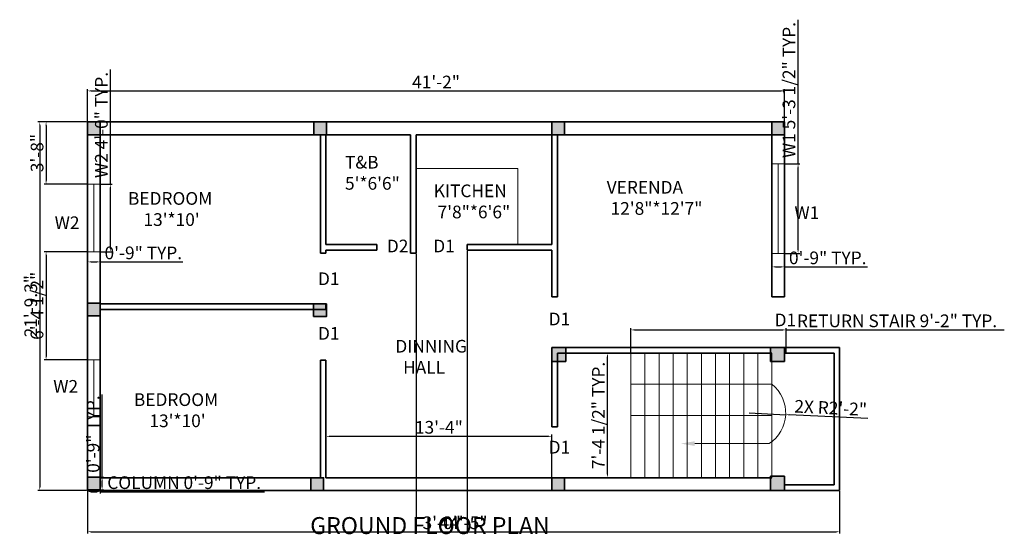
# Model space of a CAD drawing. Units: inches. Extents: x 107 to 1375, y 131 to 922.
# Tile 1 of 4: x 107 to 805, y 131 to 496. Entities that reach past the tile are written whole.
import ezdxf
from ezdxf import colors
from ezdxf.entities.mleader import LeaderData, LeaderLine
from ezdxf.math import Vec2, Vec3

# ---------------------------------------------------------------- set-up
doc = ezdxf.new("R2010")
doc.units = ezdxf.units.IN
for name, color, linetype, lineweight in [('A-ANNO-DIMS', 2, 'Continuous', 13), ('A-ANNO-TEXT', 7, 'Continuous', 18), ('A-ANNO-TITL', 7, 'Continuous', 25), ('A-AREA-IDEN', 7, 'Continuous', 18), ('A-COLS', 7, 'Continuous', 35), ('A-FLOR-FIXT', 8, 'Continuous', 18), ('A-FLOR-STRS', 7, 'Continuous', 18), ('A-GLAZ', 4, 'Continuous', 18), ('A-WALL', 7, 'Continuous', 35)]:
    doc.layers.add(name, color=color, linetype=linetype, lineweight=lineweight)
doc.layers.add('A-COLS-PATT', color=18, linetype='Continuous', lineweight=13, true_color=0x000000)
doc.styles.get("Standard").update_dxf_attribs({"font": 'arial.ttf'})
doc.dimstyles.new('ISO-25', dxfattribs={"dimtxt": 9, "dimasz": 2.5, "dimexe": 1.25, "dimexo": 0.625, "dimtad": 1, "dimlunit": 3, "dimtxsty": 'Standard', "dimcen": 2.5, "dimadec": 0, "dimazin": 0, "dimtfac": 1, "dimtmove": 0, "dimatfit": 3, "dimfxl": 1, "dimarcsym": 0})

# ---------------------------------------------------------------- blocks, each defined once
blk = doc.blocks.new('*D1')
at = {"layer": 'A-ANNO-DIMS', "color": 0, "lineweight": -2, "transparency": 16777216}
for p, q in [((155.4, 423.72), (155.4, 446.38)), ((157.9, 445.13), (646.9, 445.13)), ((649.4, 423.72), (649.4, 446.38))]:
    blk.add_line(p, q, dxfattribs=at)
at = {"layer": 'A-ANNO-DIMS', "color": 0, "transparency": 16777216}
for points in [[(157.9, 445.55), (157.9, 444.72), (155.4, 445.13)], [(646.9, 445.55), (646.9, 444.72), (649.4, 445.13)]]:
    blk.add_solid(points, dxfattribs=at)
at = {"layer": 'Defpoints', "color": 0, "transparency": 16777216}
for p in [(649.4, 445.13), (155.4, 423.09), (649.4, 423.09)]:
    blk.add_point(p, dxfattribs=at)
at = {"layer": 'A-ANNO-DIMS', "color": 0, "transparency": 16777216, "insert": (402.4, 450.28), "char_height": 9, "attachment_point": 5}
blk.add_mtext('41\'-2"', dxfattribs=at)
blk = doc.blocks.new('*D2')
at = {"layer": 'A-ANNO-DIMS', "color": 0, "lineweight": -2, "transparency": 16777216}
for p, q in [((154.77, 423.09), (120.32, 423.09)), ((121.57, 420.59), (121.57, 164.29)), ((154.77, 161.79), (120.32, 161.79))]:
    blk.add_line(p, q, dxfattribs=at)
at = {"layer": 'A-ANNO-DIMS', "color": 0, "transparency": 16777216}
for points in [[(121.15, 420.59), (121.98, 420.59), (121.57, 423.09)], [(121.15, 164.29), (121.98, 164.29), (121.57, 161.79)]]:
    blk.add_solid(points, dxfattribs=at)
at = {"layer": 'Defpoints', "color": 0, "transparency": 16777216}
for p in [(155.4, 423.09), (121.57, 161.79), (155.4, 161.79)]:
    blk.add_point(p, dxfattribs=at)
at = {"layer": 'A-ANNO-DIMS', "color": 0, "transparency": 16777216, "insert": (116.34, 292.44), "char_height": 9, "attachment_point": 5, "rotation": 90}
blk.add_mtext('21\'-9.3"', dxfattribs=at)
blk = doc.blocks.new('COLUMN-10x10')
h = blk.add_hatch(color=256)
h.dxf.hatch_style = 1
h.paths.add_polyline_path([(10, 10), (0, 10), (0, 0), (10, 0)])
for p, q in [((10, 10), (0, 10)), ((0, 10), (0, 0)), ((10, 0), (10, 10)), ((0, 0), (10, 0))]:
    blk.add_line(p, q)
blk = doc.blocks.new('COLUMN-9x9')
h = blk.add_hatch(color=256)
h.dxf.hatch_style = 1
h.paths.add_polyline_path([(9, 9), (0, 9), (0, 0), (9, 0)])
blk.add_lwpolyline([(0, 0), (9, 0), (9, 9), (0, 9)], close=True)
blk = doc.blocks.new('WINDOW-PLAN-W1')
for p, q in [((0, 63.51), (0, 0)), ((0, 63.51), (9, 63.51)), ((4.5, 63.51), (4.5, 0)), ((9, 0), (9, 63.51)), ((0, 0), (9, 0))]:
    blk.add_line(p, q)
blk = doc.blocks.new('WINDOW-PLAN-W2-OFFSET')
for p, q in [((0, 48), (0, 0)), ((0, 48), (9, 48)), ((4.5, 48), (4.5, 7.53)), ((9, 0), (9, 48)), ((0, 7.53), (9, 7.53))]:
    blk.add_line(p, q)
blk = doc.blocks.new('WINDOW-PLAN-W2')
for p, q in [((0, 48), (0, 0)), ((0, 48), (9, 48)), ((4.5, 48), (4.5, 0)), ((9, 0), (9, 48)), ((0, 0), (9, 0))]:
    blk.add_line(p, q)
blk = doc.blocks.new('KITCHEN-COUNTER-L')
for q in [(0, 54), (72, 0)]:
    blk.add_line((72, 54), q)
blk = doc.blocks.new('*D20')
at = {"layer": 'A-ANNO-DIMS', "color": 0, "lineweight": -2, "transparency": 16777216}
for p, q in [((155.4, 161.54), (155.4, 159.56)), ((157.9, 160.81), (161.9, 160.81)), ((164.4, 161.54), (164.4, 159.56)), ((164.4, 160.81), (280.88, 160.81))]:
    blk.add_line(p, q, dxfattribs=at)
at = {"layer": 'A-ANNO-DIMS', "color": 0, "transparency": 16777216}
for points in [[(157.9, 161.23), (157.9, 160.4), (155.4, 160.81)], [(161.9, 161.23), (161.9, 160.4), (164.4, 160.81)]]:
    blk.add_solid(points, dxfattribs=at)
at = {"layer": 'Defpoints', "color": 0, "transparency": 16777216}
for p in [(155.4, 162.16), (164.4, 162.16), (164.4, 160.81)]:
    blk.add_point(p, dxfattribs=at)
at = {"layer": 'A-ANNO-DIMS', "color": 0, "transparency": 16777216, "insert": (223.89, 166.1), "char_height": 9, "attachment_point": 5}
blk.add_mtext('COLUMN 0\'-9" TYP.', dxfattribs=at)
blk = doc.blocks.new('*D21')
at = {"layer": 'A-ANNO-DIMS', "color": 0, "lineweight": -2, "transparency": 16777216}
for p, q in [((165.75, 171.16), (165.75, 229.77)), ((165.02, 171.16), (167, 171.16)), ((165.75, 164.66), (165.75, 168.66)), ((165.02, 162.16), (167, 162.16))]:
    blk.add_line(p, q, dxfattribs=at)
at = {"layer": 'A-ANNO-DIMS', "color": 0, "transparency": 16777216}
for points in [[(165.33, 168.66), (166.16, 168.66), (165.75, 171.16)], [(165.33, 164.66), (166.16, 164.66), (165.75, 162.16)]]:
    blk.add_solid(points, dxfattribs=at)
at = {"layer": 'Defpoints', "color": 0, "transparency": 16777216}
for p in [(164.4, 171.16), (165.75, 171.16), (164.4, 162.16)]:
    blk.add_point(p, dxfattribs=at)
at = {"layer": 'A-ANNO-DIMS', "color": 0, "transparency": 16777216, "insert": (160.53, 201.72), "char_height": 9, "attachment_point": 5, "rotation": 90}
blk.add_mtext('0\'-9" TYP.', dxfattribs=at)
blk = doc.blocks.new('*D24')
at = {"layer": 'A-ANNO-DIMS', "color": 0, "lineweight": -2, "transparency": 16777216}
for p, q in [((658.92, 393.37), (658.92, 495.67)), ((650.02, 393.37), (660.17, 393.37)), ((658.92, 332.36), (658.92, 390.87)), ((650.02, 329.86), (660.17, 329.86))]:
    blk.add_line(p, q, dxfattribs=at)
at = {"layer": 'A-ANNO-DIMS', "color": 0, "transparency": 16777216}
for points in [[(658.51, 390.87), (659.34, 390.87), (658.92, 393.37)], [(658.51, 332.36), (659.34, 332.36), (658.92, 329.86)]]:
    blk.add_solid(points, dxfattribs=at)
at = {"layer": 'Defpoints', "color": 0, "transparency": 16777216}
for p in [(649.4, 393.37), (658.92, 393.37), (649.4, 329.86)]:
    blk.add_point(p, dxfattribs=at)
at = {"layer": 'A-ANNO-DIMS', "color": 0, "transparency": 16777216, "insert": (653.64, 445.77), "char_height": 9, "attachment_point": 5, "rotation": 90}
blk.add_mtext('W1 5\'-3 1/2" TYP.', dxfattribs=at)
blk = doc.blocks.new('*D25')
at = {"layer": 'A-ANNO-DIMS', "color": 0, "lineweight": -2, "transparency": 16777216}
for p, q in [((640.4, 329.24), (640.4, 319.09)), ((649.4, 329.24), (649.4, 319.09)), ((642.9, 320.34), (646.9, 320.34)), ((649.4, 320.34), (708.01, 320.34))]:
    blk.add_line(p, q, dxfattribs=at)
at = {"layer": 'A-ANNO-DIMS', "color": 0, "transparency": 16777216}
for points in [[(642.9, 320.75), (642.9, 319.92), (640.4, 320.34)], [(646.9, 320.75), (646.9, 319.92), (649.4, 320.34)]]:
    blk.add_solid(points, dxfattribs=at)
at = {"layer": 'Defpoints', "color": 0, "transparency": 16777216}
for p in [(640.4, 329.86), (649.4, 329.86), (649.4, 320.34)]:
    blk.add_point(p, dxfattribs=at)
at = {"layer": 'A-ANNO-DIMS', "color": 0, "transparency": 16777216, "insert": (679.95, 325.56), "char_height": 9, "attachment_point": 5}
blk.add_mtext('0\'-9" TYP.', dxfattribs=at)
blk = doc.blocks.new('*D28')
at = {"layer": 'A-ANNO-DIMS', "color": 0, "lineweight": -2, "transparency": 16777216}
for p, q in [((171.6, 379.06), (171.6, 460.39)), ((165.02, 379.06), (172.85, 379.06)), ((171.6, 333.56), (171.6, 376.56)), ((165.02, 331.06), (172.85, 331.06))]:
    blk.add_line(p, q, dxfattribs=at)
at = {"layer": 'A-ANNO-DIMS', "color": 0, "transparency": 16777216}
for points in [[(171.18, 376.56), (172.01, 376.56), (171.6, 379.06)], [(171.18, 333.56), (172.01, 333.56), (171.6, 331.06)]]:
    blk.add_solid(points, dxfattribs=at)
at = {"layer": 'Defpoints', "color": 0, "transparency": 16777216}
for p in [(164.4, 379.06), (171.6, 379.06), (164.4, 331.06)]:
    blk.add_point(p, dxfattribs=at)
at = {"layer": 'A-ANNO-DIMS', "color": 0, "transparency": 16777216, "insert": (166.38, 420.98), "char_height": 9, "attachment_point": 5, "rotation": 90}
blk.add_mtext('W2 4\'-0" TYP.', dxfattribs=at)
blk = doc.blocks.new('*D29')
at = {"layer": 'A-ANNO-DIMS', "color": 0, "lineweight": -2, "transparency": 16777216}
for p, q in [((155.4, 330.44), (155.4, 322.61)), ((164.4, 330.44), (164.4, 322.61)), ((157.9, 323.86), (161.9, 323.86)), ((164.4, 323.86), (223.01, 323.86))]:
    blk.add_line(p, q, dxfattribs=at)
at = {"layer": 'A-ANNO-DIMS', "color": 0, "transparency": 16777216}
for points in [[(157.9, 324.28), (157.9, 323.45), (155.4, 323.86)], [(161.9, 324.28), (161.9, 323.45), (164.4, 323.86)]]:
    blk.add_solid(points, dxfattribs=at)
at = {"layer": 'Defpoints', "color": 0, "transparency": 16777216}
for p in [(155.4, 331.06), (164.4, 331.06), (164.4, 323.86)]:
    blk.add_point(p, dxfattribs=at)
at = {"layer": 'A-ANNO-DIMS', "color": 0, "transparency": 16777216, "insert": (194.95, 329.08), "char_height": 9, "attachment_point": 5}
blk.add_mtext('0\'-9" TYP.', dxfattribs=at)
blk = doc.blocks.new('*D32')
at = {"layer": 'A-ANNO-DIMS', "color": 0, "lineweight": -2, "transparency": 16777216}
for p, q in [((540.4, 259.72), (540.4, 276.86)), ((542.9, 275.61), (648.03, 275.61)), ((650.53, 259.72), (650.53, 276.86)), ((650.53, 275.61), (805.07, 275.61))]:
    blk.add_line(p, q, dxfattribs=at)
at = {"layer": 'A-ANNO-DIMS', "color": 0, "transparency": 16777216}
for points in [[(542.9, 276.03), (542.9, 275.2), (540.4, 275.61)], [(648.03, 276.03), (648.03, 275.2), (650.53, 275.61)]]:
    blk.add_solid(points, dxfattribs=at)
at = {"layer": 'Defpoints', "color": 0, "transparency": 16777216}
for p in [(650.53, 275.61), (540.4, 259.09), (650.53, 259.09)]:
    blk.add_point(p, dxfattribs=at)
at = {"layer": 'A-ANNO-DIMS', "color": 0, "transparency": 16777216, "insert": (729.05, 280.89), "char_height": 9, "attachment_point": 5}
blk.add_mtext('RETURN STAIR 9\'-2" TYP.', dxfattribs=at)
blk = doc.blocks.new('*D33')
at = {"layer": 'A-ANNO-DIMS', "color": 0, "lineweight": -2, "transparency": 16777216}
for p, q in [((539.77, 259.09), (522.63, 259.09)), ((523.88, 173.29), (523.88, 256.59)), ((539.77, 170.79), (522.63, 170.79))]:
    blk.add_line(p, q, dxfattribs=at)
at = {"layer": 'A-ANNO-DIMS', "color": 0, "transparency": 16777216}
for points in [[(523.46, 256.59), (524.29, 256.59), (523.88, 259.09)], [(523.46, 173.29), (524.29, 173.29), (523.88, 170.79)]]:
    blk.add_solid(points, dxfattribs=at)
at = {"layer": 'Defpoints', "color": 0, "transparency": 16777216}
for p in [(523.88, 259.09), (540.4, 259.09), (540.4, 170.79)]:
    blk.add_point(p, dxfattribs=at)
at = {"layer": 'A-ANNO-DIMS', "color": 0, "transparency": 16777216, "insert": (518.6, 214.94), "char_height": 9, "attachment_point": 5, "rotation": 90}
blk.add_mtext('7\'-4 1/2" TYP.', dxfattribs=at)
blk = doc.blocks.new('*D46')
at = {"layer": 'A-ANNO-DIMS', "color": 0, "lineweight": -2, "transparency": 16777216}
for p, q in [((155.4, 161.17), (155.4, 131.19)), ((688.4, 161.17), (688.4, 131.19)), ((157.9, 132.44), (685.9, 132.44))]:
    blk.add_line(p, q, dxfattribs=at)
at = {"layer": 'A-ANNO-DIMS', "color": 0, "transparency": 16777216}
for points in [[(157.9, 132.86), (157.9, 132.02), (155.4, 132.44)], [(685.9, 132.86), (685.9, 132.02), (688.4, 132.44)]]:
    blk.add_solid(points, dxfattribs=at)
at = {"layer": 'Defpoints', "color": 0, "transparency": 16777216}
for p in [(155.4, 161.79), (688.4, 161.79), (688.4, 132.44)]:
    blk.add_point(p, dxfattribs=at)
at = {"layer": 'A-ANNO-DIMS', "color": 0, "transparency": 16777216, "insert": (421.9, 137.64), "char_height": 9, "attachment_point": 5}
blk.add_mtext('44\'-5"', dxfattribs=at)
blk = doc.blocks.new('*D48')
at = {"layer": 'A-ANNO-DIMS', "color": 0, "lineweight": -2, "transparency": 16777216}
for p, q in [((388.4, 329.47), (388.4, 131.19)), ((424.4, 331.47), (424.4, 131.19)), ((390.9, 132.44), (421.9, 132.44))]:
    blk.add_line(p, q, dxfattribs=at)
at = {"layer": 'A-ANNO-DIMS', "color": 0, "transparency": 16777216}
for points in [[(390.9, 132.86), (390.9, 132.02), (388.4, 132.44)], [(421.9, 132.86), (421.9, 132.02), (424.4, 132.44)]]:
    blk.add_solid(points, dxfattribs=at)
at = {"layer": 'Defpoints', "color": 0, "transparency": 16777216}
for p in [(388.4, 330.09), (424.4, 332.09), (424.4, 132.44)]:
    blk.add_point(p, dxfattribs=at)
at = {"layer": 'A-ANNO-DIMS', "color": 0, "transparency": 16777216, "insert": (406.4, 137.66), "char_height": 9, "attachment_point": 5}
blk.add_mtext('3\'-0"', dxfattribs=at)
blk = doc.blocks.new('*D49')
at = {"layer": 'A-ANNO-DIMS', "color": 0, "lineweight": -2, "transparency": 16777216}
for p, q in [((154.77, 423.09), (124.8, 423.09)), ((126.05, 420.59), (126.05, 381.56)), ((154.77, 379.06), (124.8, 379.06))]:
    blk.add_line(p, q, dxfattribs=at)
at = {"layer": 'A-ANNO-DIMS', "color": 0, "transparency": 16777216}
for points in [[(125.63, 420.59), (126.46, 420.59), (126.05, 423.09)], [(125.63, 381.56), (126.46, 381.56), (126.05, 379.06)]]:
    blk.add_solid(points, dxfattribs=at)
at = {"layer": 'Defpoints', "color": 0, "transparency": 16777216}
for p in [(155.4, 423.09), (126.05, 379.06), (155.4, 379.06)]:
    blk.add_point(p, dxfattribs=at)
at = {"layer": 'A-ANNO-DIMS', "color": 0, "transparency": 16777216, "insert": (120.82, 401.08), "char_height": 9, "attachment_point": 5, "rotation": 90}
blk.add_mtext('3\'-8"', dxfattribs=at)
blk = doc.blocks.new('*D50')
at = {"layer": 'A-ANNO-DIMS', "color": 0, "lineweight": -2, "transparency": 16777216}
for p, q in [((154.77, 331.06), (124.8, 331.06)), ((126.05, 328.56), (126.05, 256.86)), ((154.77, 254.36), (124.8, 254.36))]:
    blk.add_line(p, q, dxfattribs=at)
at = {"layer": 'A-ANNO-DIMS', "color": 0, "transparency": 16777216}
for points in [[(125.63, 328.56), (126.46, 328.56), (126.05, 331.06)], [(125.63, 256.86), (126.46, 256.86), (126.05, 254.36)]]:
    blk.add_solid(points, dxfattribs=at)
at = {"layer": 'Defpoints', "color": 0, "transparency": 16777216}
for p in [(155.4, 331.06), (126.05, 254.36), (155.4, 254.36)]:
    blk.add_point(p, dxfattribs=at)
at = {"layer": 'A-ANNO-DIMS', "color": 0, "transparency": 16777216, "insert": (120.77, 292.71), "char_height": 9, "attachment_point": 5, "rotation": 90}
blk.add_mtext('6\'-4 1/2"', dxfattribs=at)
blk = doc.blocks.new('*D55')
at = {"layer": 'A-ANNO-DIMS', "color": 0, "lineweight": -2, "transparency": 16777216}
for p, q in [((324.4, 171.42), (324.4, 201.39)), ((326.9, 200.14), (481.9, 200.14)), ((484.4, 171.42), (484.4, 201.39))]:
    blk.add_line(p, q, dxfattribs=at)
at = {"layer": 'A-ANNO-DIMS', "color": 0, "transparency": 16777216}
for points in [[(326.9, 200.56), (326.9, 199.72), (324.4, 200.14)], [(481.9, 200.56), (481.9, 199.72), (484.4, 200.14)]]:
    blk.add_solid(points, dxfattribs=at)
at = {"layer": 'Defpoints', "color": 0, "transparency": 16777216}
for p in [(484.4, 200.14), (324.4, 170.79), (484.4, 170.79)]:
    blk.add_point(p, dxfattribs=at)
at = {"layer": 'A-ANNO-DIMS', "color": 0, "transparency": 16777216, "insert": (404.4, 205.36), "char_height": 9, "attachment_point": 5}
blk.add_mtext('13\'-4"', dxfattribs=at)
blk = doc.blocks.new('*D79')
at = {"layer": 'A-ANNO-DIMS', "color": 0, "lineweight": -2, "transparency": 16777216}
for p, q in [((624.18, 216.72), (650.14, 215.49)), ((708.35, 212.72), (652.63, 215.37))]:
    blk.add_line(p, q, dxfattribs=at)
at = {"layer": 'A-ANNO-DIMS', "color": 0, "transparency": 16777216}
blk.add_solid([(652.65, 215.79), (652.61, 214.95), (650.14, 215.49)], dxfattribs=at)
at = {"layer": 'Defpoints', "color": 0, "transparency": 16777216}
for p in [(624.18, 216.72), (650.14, 215.49)]:
    blk.add_point(p, dxfattribs=at)
at = {"layer": 'A-ANNO-DIMS', "color": 0, "transparency": 16777216, "insert": (681.99, 219.13), "char_height": 9, "attachment_point": 5, "rotation": 357.27702}
blk.add_mtext('2X R2\'-2"', dxfattribs=at)
blk = doc.blocks.new('STAIR-RETURN-PLAN')
for p, q in [((0, 0), (0, 88.3)), ((10, 0), (10, 88.3)), ((20, 0), (20, 88.3)), ((30, 0), (30, 88.3)), ((40, 0), (40, 88.3)), ((50, 0), (50, 88.3)), ((60, 0), (60, 88.3)), ((70, 0), (70, 88.3)), ((80, 0), (80, 88.3)), ((90, 0), (90, 88.3)), ((100, 0), (100, 88.3)), ((0, 66.24), (100, 66.24)), ((0, 44.15), (100, 44.15))]:
    blk.add_line(p, q)
for start, end in [(303.16419, 51.39065), (236.83581, 237.96095)]:
    blk.add_arc((83.79, 45.93), 25.99, start, end)
ml = blk.add_multileader_mtext('Standard')
ml.set_content('', color=256)
ml.set_leader_properties(color=256)
ml.build(insert=Vec2(0, 0))
ml.multileader.update_dxf_attribs({"arrow_head_size": 10})
ctx = ml.context
ctx.base_point, ctx.arrow_head_size, ctx.plane_origin = Vec3(98, 24.18), 10, Vec3(35.35, 24.18)
notes = []
notes.append((ctx, [(0, (1, 1, 0), (90, 24.18), (1, 0), 8, [(0, [(35.35, 24.18)], 0, [])])]))
ctx.mtext.insert, ctx.mtext.flow_direction = Vec3(100, 26.18), 5
for ctx, leaders in notes:
    for number, flags, end, landing, length, lines in leaders:
        leader = LeaderData()
        leader.index, (leader.has_last_leader_line, leader.has_dogleg_vector, leader.attachment_direction) = number, flags
        leader.last_leader_point, leader.dogleg_vector, leader.dogleg_length = Vec3(end), Vec3(landing), length
        for number, points, colour, breaks in lines:
            line = LeaderLine()
            line.index, line.vertices, line.color, line.breaks = number, Vec3.list(points), colors.encode_raw_color(colour), breaks
            leader.lines.append(line)
        ctx.leaders.append(leader)

msp = doc.modelspace()

# ---------------------------------------------------------------- hatches: boundary and pattern name
at = {"layer": 'A-COLS-PATT'}
h = msp.add_hatch(color=256, dxfattribs=at)
h.dxf.hatch_style = 1
h.paths.add_polyline_path([(164.397, 423.091), (155.397, 423.091), (155.397, 414.091), (164.397, 414.091)])

# ---------------------------------------------------------------- linework, layer by layer
at = {"layer": 'A-COLS'}
msp.add_lwpolyline([(155.397, 414.091), (164.397, 414.091), (164.397, 423.091), (155.397, 423.091)], close=True, dxfattribs=at)
at = {"layer": 'A-WALL'}
for p, q in [((649.397, 423.091), (155.397, 423.091)), ((155.397, 423.091), (155.397, 161.791)), ((649.397, 299.091), (649.397, 423.091)), ((164.397, 414.091), (164.397, 294.091)), ((320.397, 414.091), (164.397, 414.091)), ((320.397, 414.091), (320.397, 330.091)), ((324.397, 414.091), (324.397, 336.091)), ((384.397, 414.091), (324.397, 414.091)), ((384.397, 414.091), (384.397, 330.091)), ((402.397, 414.091), (388.397, 414.091)), ((484.397, 414.091), (388.397, 414.091)), ((388.397, 414.091), (388.397, 330.091)), ((484.397, 414.091), (484.397, 336.091)), ((640.397, 414.091), (488.397, 414.091)), ((488.397, 414.091), (488.397, 299.091)), ((640.397, 299.091), (640.397, 414.091)), ((360.397, 336.091), (324.397, 336.091)), ((360.397, 336.091), (360.397, 332.091)), ((484.397, 336.091), (424.397, 336.091)), ((424.397, 336.091), (424.397, 332.091)), ((320.397, 330.091), (324.397, 330.091)), ((360.397, 332.091), (324.397, 332.091)), ((324.397, 332.091), (324.397, 330.091)), ((384.397, 330.091), (388.397, 330.091)), ((484.397, 332.091), (424.397, 332.091)), ((484.397, 332.091), (484.397, 299.091)), ((324.397, 294.091), (164.397, 294.091)), ((324.397, 294.091), (324.397, 290.091)), ((488.397, 299.091), (484.397, 299.091)), ((640.397, 299.091), (649.397, 299.091)), ((324.397, 290.091), (164.397, 290.091)), ((164.397, 290.091), (164.397, 170.791)), ((640.397, 263.091), (484.397, 263.091)), ((484.397, 263.091), (484.397, 206.791)), ((640.397, 259.091), (488.397, 259.091)), ((488.397, 259.091), (488.397, 206.791)), ((640.397, 263.091), (688.397, 263.091)), ((649.319, 263.091), (649.319, 259.091)), ((649.319, 259.091), (684.397, 259.091)), ((684.397, 259.091), (684.397, 165.791)), ((688.397, 263.091), (688.397, 161.791)), ((324.397, 254.091), (320.397, 254.091)), ((320.397, 254.091), (320.397, 170.791)), ((324.397, 254.091), (324.397, 170.791)), ((484.397, 206.791), (488.397, 206.791)), ((164.397, 170.791), (320.397, 170.791)), ((324.397, 170.791), (640.397, 170.791)), ((155.397, 161.791), (649.397, 161.791)), ((684.397, 165.791), (649.397, 165.791)), ((649.397, 165.791), (649.397, 161.791)), ((688.397, 161.791), (649.397, 161.791))]:
    msp.add_line(p, q, dxfattribs=at)

# ---------------------------------------------------------------- block references
at = {"layer": 'A-COLS'}
for name, p in [('COLUMN-9x9', (315.721, 414.091)), ('COLUMN-9x9', (484.336, 414.091)), ('COLUMN-9x9', (640.354, 414.091)), ('COLUMN-9x9', (155.397, 285.58)), ('COLUMN-9x9', (315.659, 285.091)), ('COLUMN-10x10', (484.397, 253.091)), ('COLUMN-10x10', (639.319, 253.091)), ('COLUMN-9x9', (155.397, 162.165)), ('COLUMN-9x9', (313.71, 161.791)), ('COLUMN-9x9', (484.397, 161.791)), ('COLUMN-10x10', (639.397, 161.791))]:
    msp.add_blockref(name, p, dxfattribs=at)
at = {"layer": 'A-FLOR-FIXT'}
msp.add_blockref('KITCHEN-COUNTER-L', (388.397, 336.091), dxfattribs=at)
at = {"layer": 'A-FLOR-STRS'}
msp.add_blockref('STAIR-RETURN-PLAN', (540.397, 170.791), dxfattribs=at)
at = {"layer": 'A-GLAZ'}
for name, p in [('WINDOW-PLAN-W1', (640.397, 329.862)), ('WINDOW-PLAN-W2', (155.397, 331.064)), ('WINDOW-PLAN-W2-OFFSET', (155.397, 206.359))]:
    msp.add_blockref(name, p, dxfattribs=at)

# ---------------------------------------------------------------- texts
at = {"layer": 'A-ANNO-TEXT', "char_height": 9, "attachment_point": 1}
for s, insert in [('W1', (656.351, 363.214)), ('W2', (132.141, 356.135)), ('D2', (367.525, 339.617)), ('D1', (400.427, 339.617)), ('D1', (318.726, 316.377)), ('D1', (482.182, 287.865)), ('D1', (642.301, 287.194)), ('D1', (318.726, 277.637)), ('W2', (131.147, 240.071)), ('D1', (482.182, 196.943))]:
    msp.add_mtext_dynamic_manual_height_columns(s, width=33.2577, gutter_width=12.5, heights=[0], dxfattribs=dict(at, insert=insert))
at = {"layer": 'A-ANNO-TITL', "insert": (313.216, 142.83), "char_height": 12, "attachment_point": 1}
msp.add_mtext_dynamic_manual_height_columns('GROUND FLOOR PLAN', width=264.80934, gutter_width=12.5, heights=[0], dxfattribs=at)
at = {"layer": 'A-AREA-IDEN', "char_height": 9, "attachment_point": 1}
for s, width, insert in [('T&B\\P5\'*6\'6"', 26.62767, (337.879, 399.061)), ('KITCHEN\\P 7\'8"*6\'6"', 54.9024, (400.742, 378.764)), ('VERENDA \\P 12\'8"*12\'7"', 89.49012, (523.321, 381.268)), ("BEDROOM\\P    13'*10'", 64.41797, (184.073, 373.369)), ('DINNING\\P  HALL ', 53.67099, (373.54, 268.537)), ("BEDROOM\\P    13'*10'", 64.41797, (188.274, 230.643))]:
    msp.add_mtext_dynamic_manual_height_columns(s, width=width, gutter_width=12.5, heights=[0], dxfattribs=dict(at, insert=insert))

# ---------------------------------------------------------------- dimensions: what is measured, and where the dimension line sits
at = {"layer": 'A-ANNO-DIMS'}
for base, p1, p2, text, picture, middle in [((658.923, 393.37), (649.397, 329.862), (649.397, 393.37), 'W1 <> TYP.', '*D24', (653.641, 445.771)), ((171.597, 379.064), (164.397, 331.064), (164.397, 379.064), 'W2 <> TYP.', '*D28', (166.377, 420.979)), ((523.876, 259.091), (540.397, 170.791), (540.397, 259.091), '<> TYP.', '*D33', (518.598, 214.941)), ((165.747, 171.165), (164.397, 162.165), (164.397, 171.165), '<> TYP.', '*D21', (160.527, 201.72))]:
    dim = msp.add_linear_dim(base=base, p1=p1, p2=p2, angle=90, text=text, dimstyle='ISO-25', override={"dimdec": 1, "dimlfac": 1, "dimrnd": 0, "dimzin": 1, "dimdsep": 46, "dimlunit": 4, "dimfrac": 2}, dxfattribs=at)
    dim.commit()
    dim.dimension.update_dxf_attribs({"geometry": picture, "text_midpoint": middle})
for base, p1, p2, override, picture, middle in [((649.397, 445.133), (155.397, 423.091), (649.397, 423.091), {"dimclrd": 0, "dimclre": 0, "dimclrt": 0}, '*D1', (402.397, 450.276)), ((424.397, 132.441), (388.397, 330.091), (424.397, 332.091), {"dimdec": 1, "dimlfac": 1, "dimrnd": 0, "dimzin": 1, "dimdsep": 46, "dimlunit": 4, "dimfrac": 2}, '*D48', (406.397, 137.665)), ((688.397, 132.441), (155.397, 161.791), (688.397, 161.791), {"dimdec": 1, "dimlfac": 1, "dimrnd": 0, "dimzin": 1, "dimdsep": 46, "dimlunit": 4, "dimfrac": 2}, '*D46', (421.897, 137.643))]:
    dim = msp.add_linear_dim(base=base, p1=p1, p2=p2, dimstyle='ISO-25', override=override, dxfattribs=at)
    dim.commit()
    dim.dimension.update_dxf_attribs({"geometry": picture, "text_midpoint": middle})
for base, p1, p2, angle, override, picture, middle in [((121.568, 161.791), (155.397, 423.091), (155.397, 161.791), 90, {"dimclrd": 0, "dimclre": 0, "dimclrt": 0}, '*D2', (116.345, 292.441)), ((126.047, 379.064), (155.397, 423.091), (155.397, 379.064), 90, {"dimdec": 1, "dimlfac": 1, "dimrnd": 0, "dimzin": 1, "dimdsep": 46, "dimlunit": 4, "dimfrac": 2}, '*D49', (120.823, 401.078)), ((126.047, 254.359), (155.397, 331.064), (155.397, 254.359), 90, {"dimdec": 1, "dimlfac": 1, "dimrnd": 0, "dimzin": 1, "dimdsep": 46, "dimlunit": 4, "dimfrac": 2}, '*D50', (120.768, 292.712)), ((484.397, 200.141), (324.397, 170.791), (484.397, 170.791), 0, {"dimdec": 1, "dimlfac": 1, "dimrnd": 0, "dimzin": 1, "dimdsep": 46, "dimlunit": 4, "dimfrac": 2}, '*D55', (404.397, 205.365))]:
    dim = msp.add_linear_dim(base=base, p1=p1, p2=p2, angle=angle, dimstyle='ISO-25', override=override, dxfattribs=at)
    dim.commit()
    dim.dimension.update_dxf_attribs({"geometry": picture, "text_midpoint": middle})
for base, p1, p2, text, picture, middle in [((164.397, 323.864), (155.397, 331.064), (164.397, 331.064), '<> TYP.', '*D29', (194.951, 329.084)), ((649.397, 320.336), (640.397, 329.862), (649.397, 329.862), '<> TYP.', '*D25', (679.951, 325.556)), ((650.534, 275.612), (540.397, 259.091), (650.534, 259.091), 'RETURN STAIR <> TYP.', '*D32', (729.054, 280.89)), ((164.397, 160.815), (155.397, 162.165), (164.397, 162.165), 'COLUMN <> TYP.', '*D20', (223.888, 166.096))]:
    dim = msp.add_linear_dim(base=base, p1=p1, p2=p2, text=text, dimstyle='ISO-25', override={"dimdec": 1, "dimlfac": 1, "dimrnd": 0, "dimzin": 1, "dimdsep": 46, "dimlunit": 4, "dimfrac": 2}, dxfattribs=at)
    dim.commit()
    dim.dimension.update_dxf_attribs({"geometry": picture, "text_midpoint": middle})
dim = msp.add_radius_dim(center=(624.182, 216.722), mpoint=(650.138, 215.488), text='2X <>', dimstyle='ISO-25', override={"dimdec": 1, "dimlfac": 1, "dimrnd": 0, "dimzin": 1, "dimdsep": 46, "dimlunit": 4, "dimfrac": 2}, dxfattribs=at)
dim.commit()
dim.dimension.update_dxf_attribs({"geometry": '*D79', "text_midpoint": (681.986, 219.126)})

doc.saveas('drawing.dxf')
